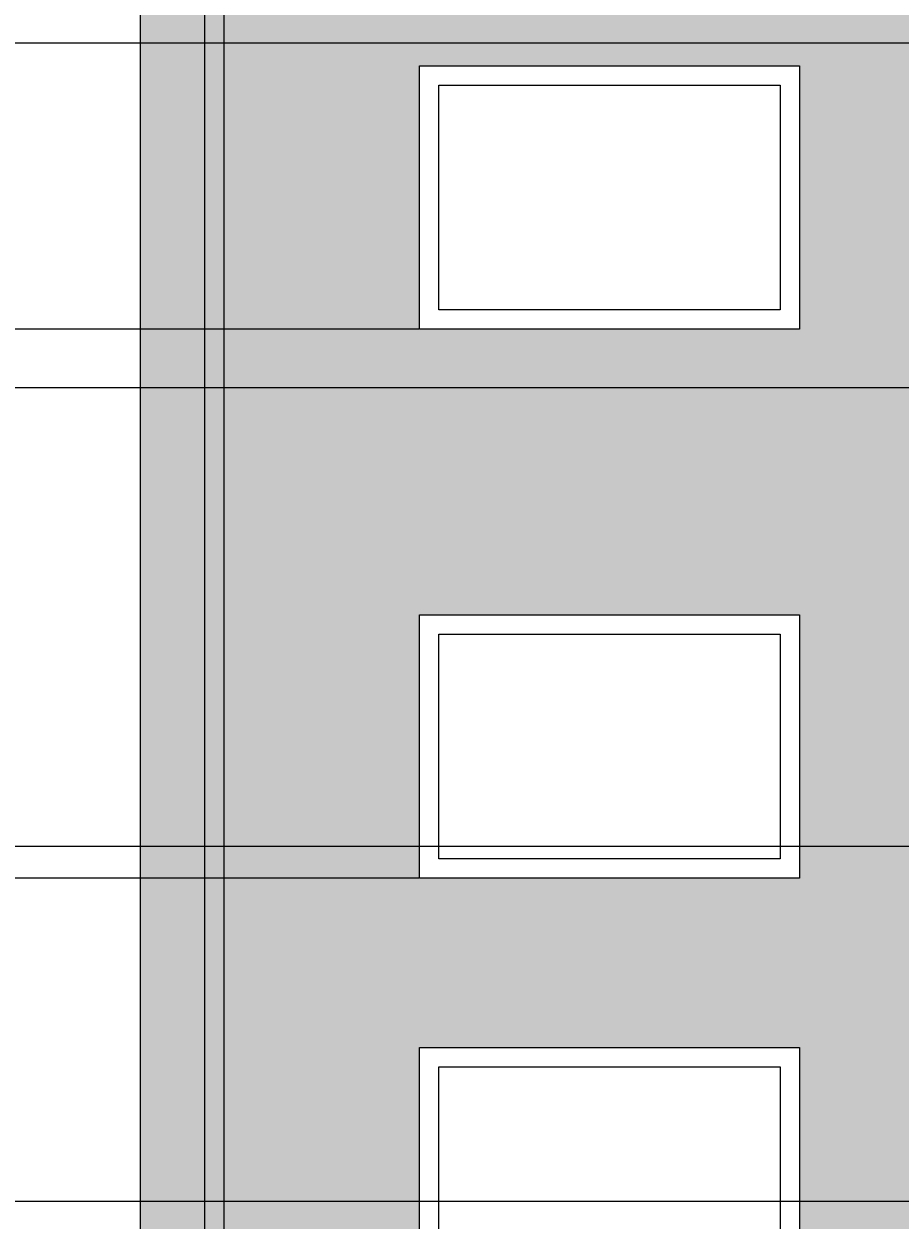
# Model space of a CAD drawing. Units: inches. Extents: x -13 to 809, y 112 to 656.
# Tile 25 of 55: x 430 to 521, y 323 to 446. Entities that reach past the tile are written whole.
import ezdxf

# ---------------------------------------------------------------- set-up
doc = ezdxf.new("R2010")
doc.units = ezdxf.units.IN
doc.header["$MEASUREMENT"] = 0
for name, color, linetype, lineweight in [('A-ANNO-DIMS', 2, 'Continuous', 18), ('A-ELEV-PATT', 8, 'Continuous', 13), ('A-GLAZ', 4, 'Continuous', 25)]:
    doc.layers.add(name, color=color, linetype=linetype, lineweight=lineweight)
doc.styles.get("Standard").update_dxf_attribs({"font": 'arial.ttf'})
doc.dimstyles.get("Standard").update_dxf_attribs({"dimtxt": 0.625, "dimasz": 0.18, "dimexe": 0.18, "dimexo": 0.0625, "dimgap": 0.09, "dimtad": 0, "dimtih": 1, "dimtoh": 1, "dimdec": 4, "dimzin": 0, "dimdsep": 46, "dimlunit": 4, "dimtxsty": 'Standard', "dimcen": 0.09, "dimadec": 0, "dimazin": 0, "dimtfac": 1, "dimtdec": 4, "dimtofl": 0, "dimtmove": 0, "dimatfit": 3, "dimfxl": 1, "dimtolj": 1, "dimtzin": 0, "dimarcsym": 0})

# ---------------------------------------------------------------- blocks, each defined once
blk = doc.blocks.new('WIN-FIXED-400')
for points in [[(0, 27.27), (39.36, 27.27), (39.36, 0), (0, 0)], [(2, 25.27), (37.36, 25.27), (37.36, 2), (2, 2)]]:
    blk.add_lwpolyline(points, close=True)
blk = doc.blocks.new('*D41')
at = {"layer": 'A-ANNO-DIMS', "color": 0, "lineweight": -2, "transparency": 16777216}
for p, q in [((471.04, 357.98), (-12.1, 357.98)), ((-11.92, 357.8), (-11.92, 335.98)), ((-11.92, 313.35), (-11.92, 335.16)), ((471.04, 313.17), (-12.1, 313.17))]:
    blk.add_line(p, q, dxfattribs=at)
at = {"layer": 'A-ANNO-DIMS', "color": 0, "transparency": 16777216}
for points in [[(-11.95, 357.8), (-11.89, 357.8), (-11.92, 357.98)], [(-11.95, 313.35), (-11.89, 313.35), (-11.92, 313.17)]]:
    blk.add_solid(points, dxfattribs=at)
at = {"layer": 'Defpoints', "color": 0, "transparency": 16777216}
for p in [(-11.92, 357.98), (471.1, 357.98), (471.1, 313.17)]:
    blk.add_point(p, dxfattribs=at)
at = {"layer": 'A-ANNO-DIMS', "color": 0, "transparency": 16777216, "insert": (-11.92, 335.57), "char_height": 0.625, "attachment_point": 5}
blk.add_mtext('\\A1;44.81', dxfattribs=at)
blk = doc.blocks.new('*D42')
at = {"layer": 'A-ANNO-DIMS', "color": 0, "lineweight": -2, "transparency": 16777216}
for p, q in [((471.04, 414.86), (-12.1, 414.86)), ((-11.92, 414.68), (-11.92, 386.83)), ((-11.92, 358.16), (-11.92, 386.01)), ((471.04, 357.98), (-12.1, 357.98))]:
    blk.add_line(p, q, dxfattribs=at)
at = {"layer": 'A-ANNO-DIMS', "color": 0, "transparency": 16777216}
for points in [[(-11.95, 414.68), (-11.89, 414.68), (-11.92, 414.86)], [(-11.95, 358.16), (-11.89, 358.16), (-11.92, 357.98)]]:
    blk.add_solid(points, dxfattribs=at)
at = {"layer": 'Defpoints', "color": 0, "transparency": 16777216}
for p in [(-11.92, 414.86), (471.1, 414.86), (471.1, 357.98)]:
    blk.add_point(p, dxfattribs=at)
at = {"layer": 'A-ANNO-DIMS', "color": 0, "transparency": 16777216, "insert": (-11.92, 386.42), "char_height": 0.625, "attachment_point": 5}
blk.add_mtext('\\A1;56.88', dxfattribs=at)
blk = doc.blocks.new('*D43')
at = {"layer": 'A-ANNO-DIMS', "color": 0, "lineweight": -2, "transparency": 16777216}
for p, q in [((471.04, 470.88), (-12.1, 470.88)), ((-11.92, 470.7), (-11.92, 443.28)), ((-11.92, 415.04), (-11.92, 442.46)), ((471.04, 414.86), (-12.1, 414.86))]:
    blk.add_line(p, q, dxfattribs=at)
at = {"layer": 'A-ANNO-DIMS', "color": 0, "transparency": 16777216}
for points in [[(-11.95, 470.7), (-11.89, 470.7), (-11.92, 470.88)], [(-11.95, 415.04), (-11.89, 415.04), (-11.92, 414.86)]]:
    blk.add_solid(points, dxfattribs=at)
at = {"layer": 'Defpoints', "color": 0, "transparency": 16777216}
for p in [(-11.92, 470.88), (471.1, 470.88), (471.1, 414.86)]:
    blk.add_point(p, dxfattribs=at)
at = {"layer": 'A-ANNO-DIMS', "color": 0, "transparency": 16777216, "insert": (-11.92, 442.87), "char_height": 0.625, "attachment_point": 5}
blk.add_mtext('\\A1;56.02', dxfattribs=at)
blk = doc.blocks.new('*D46')
at = {"layer": 'A-ANNO-DIMS', "color": 0, "lineweight": -2, "transparency": 16777216}
for p, q in [((160.98, 408.79), (807.77, 408.79)), ((807.59, 408.61), (807.59, 367.07)), ((807.59, 324.7), (807.59, 366.25)), ((160.98, 324.52), (807.77, 324.52))]:
    blk.add_line(p, q, dxfattribs=at)
at = {"layer": 'A-ANNO-DIMS', "color": 0, "transparency": 16777216}
for points in [[(807.56, 408.61), (807.62, 408.61), (807.59, 408.79)], [(807.56, 324.7), (807.62, 324.7), (807.59, 324.52)]]:
    blk.add_solid(points, dxfattribs=at)
at = {"layer": 'Defpoints', "color": 0, "transparency": 16777216}
for p in [(160.92, 408.79), (807.59, 408.79), (160.92, 324.52)]:
    blk.add_point(p, dxfattribs=at)
at = {"layer": 'A-ANNO-DIMS', "color": 0, "transparency": 16777216, "insert": (807.59, 366.66), "char_height": 0.625, "attachment_point": 5}
blk.add_mtext('\\A1;84.27', dxfattribs=at)
blk = doc.blocks.new('*D47')
at = {"layer": 'A-ANNO-DIMS', "color": 0, "lineweight": -2, "transparency": 16777216}
for p, q in [((275.78, 408.79), (807.77, 408.79)), ((807.59, 408.61), (807.59, 385.45)), ((807.59, 361.47), (807.59, 384.63)), ((275.78, 361.29), (807.77, 361.29))]:
    blk.add_line(p, q, dxfattribs=at)
at = {"layer": 'A-ANNO-DIMS', "color": 0, "transparency": 16777216}
for points in [[(807.56, 408.61), (807.62, 408.61), (807.59, 408.79)], [(807.56, 361.47), (807.62, 361.47), (807.59, 361.29)]]:
    blk.add_solid(points, dxfattribs=at)
at = {"layer": 'Defpoints', "color": 0, "transparency": 16777216}
for p in [(275.71, 408.79), (807.59, 408.79), (275.71, 361.29)]:
    blk.add_point(p, dxfattribs=at)
at = {"layer": 'A-ANNO-DIMS', "color": 0, "transparency": 16777216, "insert": (807.59, 385.04), "char_height": 0.625, "attachment_point": 5}
blk.add_mtext('\\A1;47.5', dxfattribs=at)
blk = doc.blocks.new('*D48')
at = {"layer": 'A-ANNO-DIMS', "color": 0, "lineweight": -2, "transparency": 16777216}
for p, q in [((319.57, 444.52), (807.77, 444.52)), ((807.59, 444.34), (807.59, 384.93)), ((807.59, 324.7), (807.59, 384.11)), ((319.57, 324.52), (807.77, 324.52))]:
    blk.add_line(p, q, dxfattribs=at)
at = {"layer": 'A-ANNO-DIMS', "color": 0, "transparency": 16777216}
for points in [[(807.56, 444.34), (807.62, 444.34), (807.59, 444.52)], [(807.56, 324.7), (807.62, 324.7), (807.59, 324.52)]]:
    blk.add_solid(points, dxfattribs=at)
at = {"layer": 'Defpoints', "color": 0, "transparency": 16777216}
for p in [(319.51, 444.52), (807.59, 444.52), (319.51, 324.52)]:
    blk.add_point(p, dxfattribs=at)
at = {"layer": 'A-ANNO-DIMS', "color": 0, "transparency": 16777216, "insert": (807.59, 384.52), "char_height": 0.625, "attachment_point": 5}
blk.add_mtext('\\A1;120', dxfattribs=at)
blk = doc.blocks.new('*D105')
at = {"layer": 'A-ANNO-DIMS', "color": 0, "lineweight": -2, "transparency": 16777216}
for p, q in [((319.76, 452.56), (807.77, 452.56)), ((807.59, 452.38), (807.59, 448.95)), ((807.59, 444.7), (807.59, 448.13)), ((319.57, 444.52), (807.77, 444.52))]:
    blk.add_line(p, q, dxfattribs=at)
at = {"layer": 'A-ANNO-DIMS', "color": 0, "transparency": 16777216}
for points in [[(807.56, 452.38), (807.62, 452.38), (807.59, 452.56)], [(807.56, 444.7), (807.62, 444.7), (807.59, 444.52)]]:
    blk.add_solid(points, dxfattribs=at)
at = {"layer": 'Defpoints', "color": 0, "transparency": 16777216}
for p in [(319.7, 452.56), (319.51, 444.52), (807.59, 444.52)]:
    blk.add_point(p, dxfattribs=at)
at = {"layer": 'A-ANNO-DIMS', "color": 0, "transparency": 16777216, "insert": (807.59, 448.54), "char_height": 0.625, "attachment_point": 5}
blk.add_mtext('\\A1;8.043', dxfattribs=at)
blk = doc.blocks.new('*D133')
at = {"layer": 'A-ANNO-DIMS', "color": 0, "lineweight": -2, "transparency": 16777216}
for p, q in [((448.701738, 655.782835), (448.521738, 655.782835)), ((448.881738, 207.535185), (448.881738, 655.962835)), ((450.881738, 207.527657), (450.881738, 655.962835)), ((451.061738, 655.782835), (451.241738, 655.782835))]:
    blk.add_line(p, q, dxfattribs=at)
at = {"layer": 'A-ANNO-DIMS', "color": 0, "transparency": 16777216}
for points in [[(448.701738, 655.812835), (448.701738, 655.752835), (448.881738, 655.782835)], [(451.061738, 655.812835), (451.061738, 655.752835), (450.881738, 655.782835)]]:
    blk.add_solid(points, dxfattribs=at)
at = {"layer": 'Defpoints', "color": 0, "transparency": 16777216}
for p in [(450.881738, 655.782835), (448.881738, 207.472685), (450.881738, 207.465157)]:
    blk.add_point(p, dxfattribs=at)
at = {"layer": 'A-ANNO-DIMS', "color": 0, "transparency": 16777216, "insert": (449.881738, 655.782835), "char_height": 0.625, "attachment_point": 5}
blk.add_mtext('\\A1;2.00', dxfattribs=at)

msp = doc.modelspace()

# ---------------------------------------------------------------- hatches: boundary and pattern name
at = {"layer": 'A-ELEV-PATT'}
h = msp.add_hatch(dxfattribs=at)
h.set_pattern_fill('CROSS', color=256, scale=9.7)
h.paths.add_polyline_path([(542.9617, 524.281), (442.1845, 524.281), (442.1845, 288.4508), (542.9617, 288.4508)])
h.paths.add_polyline_path([(471.0998, 470.8765), (471.0998, 498.1452), (510.462, 498.1452), (510.462, 470.8765)], flags=16)
h.paths.add_polyline_path([(473.0998, 472.8765), (473.0998, 496.1452), (508.462, 496.1452), (508.462, 472.8765)], flags=0)
h.paths.add_polyline_path([(471.0998, 442.128), (510.462, 442.128), (510.462, 414.8594), (471.0998, 414.8594)], flags=16)
h.paths.add_polyline_path([(473.0998, 440.128), (508.462, 440.128), (508.462, 416.8594), (473.0998, 416.8594)], flags=0)
h.paths.add_polyline_path([(471.0998, 385.2491), (510.462, 385.2491), (510.462, 357.9804), (471.0998, 357.9804)], flags=16)
h.paths.add_polyline_path([(473.0998, 383.2491), (508.462, 383.2491), (508.462, 359.9804), (473.0998, 359.9804)], flags=0)
h.paths.add_polyline_path([(471.0998, 340.4353), (510.462, 340.4353), (510.462, 313.1667), (471.0998, 313.1667)], flags=16)
h.paths.add_polyline_path([(473.0998, 338.4353), (508.462, 338.4353), (508.462, 315.1667), (473.0998, 315.1667)], flags=0)

# ---------------------------------------------------------------- linework, layer by layer
msp.add_line((442.1845, 524.281), (442.1845, 288.4508), dxfattribs=at)

# ---------------------------------------------------------------- block references
at = {"layer": 'A-GLAZ'}
for p in [(471.1, 414.8598), (471.1, 357.9809), (471.1, 313.1672)]:
    msp.add_blockref('WIN-FIXED-400', p, dxfattribs=at)

# ---------------------------------------------------------------- dimensions: what is measured, and where the dimension line sits
at = {"layer": 'A-ANNO-DIMS'}
dim = msp.add_linear_dim(base=(450.8817, 655.7828), p1=(448.8817, 207.4727), p2=(450.8817, 207.4652), dimstyle='Standard', override={"dimdec": 2, "dimlfac": 1, "dimrnd": 0, "dimzin": 0, "dimdsep": 46, "dimlunit": 2}, dxfattribs=at)
dim.commit()
dim.dimension.update_dxf_attribs({"geometry": '*D133', "text_midpoint": (449.8817, 655.7828)})
for base, p1, p2, override, picture, middle in [((-11.9191, 470.8765), (471.0998, 414.8594), (471.0998, 470.8765), {"dimdec": 2, "dimlfac": 1, "dimrnd": 0, "dimzin": 0, "dimdsep": 46, "dimlunit": 2}, '*D43', (-11.9191, 442.8679)), ((807.5888, 444.5199), (319.7004, 452.5629), (319.5074, 444.5199), {"dimdec": 3, "dimlfac": 1, "dimrnd": 0, "dimzin": 0, "dimdsep": 46, "dimlunit": 2}, '*D105', (807.5888, 448.5414)), ((807.5888, 444.5199), (319.5074, 324.5199), (319.5074, 444.5199), {"dimdec": 0, "dimlfac": 1, "dimrnd": 0, "dimzin": 0, "dimdsep": 46, "dimlunit": 2}, '*D48', (807.5888, 384.5199)), ((-11.9191, 414.8594), (471.0998, 357.9804), (471.0998, 414.8594), {"dimdec": 2, "dimlfac": 1, "dimrnd": 0, "dimzin": 0, "dimdsep": 46, "dimlunit": 2}, '*D42', (-11.9191, 386.4199)), ((807.5888, 408.7939), (160.9184, 324.5199), (160.9184, 408.7939), {"dimdec": 2, "dimlfac": 1, "dimrnd": 0, "dimzin": 0, "dimdsep": 46, "dimlunit": 2}, '*D46', (807.5888, 366.6569)), ((807.5888, 408.7939), (275.7145, 361.2915), (275.7145, 408.7939), {"dimdec": 1, "dimlfac": 1, "dimrnd": 0, "dimzin": 0, "dimdsep": 46, "dimlunit": 2}, '*D47', (807.5888, 385.0427)), ((-11.9191, 357.9804), (471.0998, 313.1667), (471.0998, 357.9804), {"dimdec": 2, "dimlfac": 1, "dimrnd": 0, "dimzin": 0, "dimdsep": 46, "dimlunit": 2}, '*D41', (-11.9191, 335.5735))]:
    dim = msp.add_linear_dim(base=base, p1=p1, p2=p2, angle=90, dimstyle='Standard', override=override, dxfattribs=at)
    dim.commit()
    dim.dimension.update_dxf_attribs({"geometry": picture, "text_midpoint": middle})

doc.saveas('drawing.dxf')
